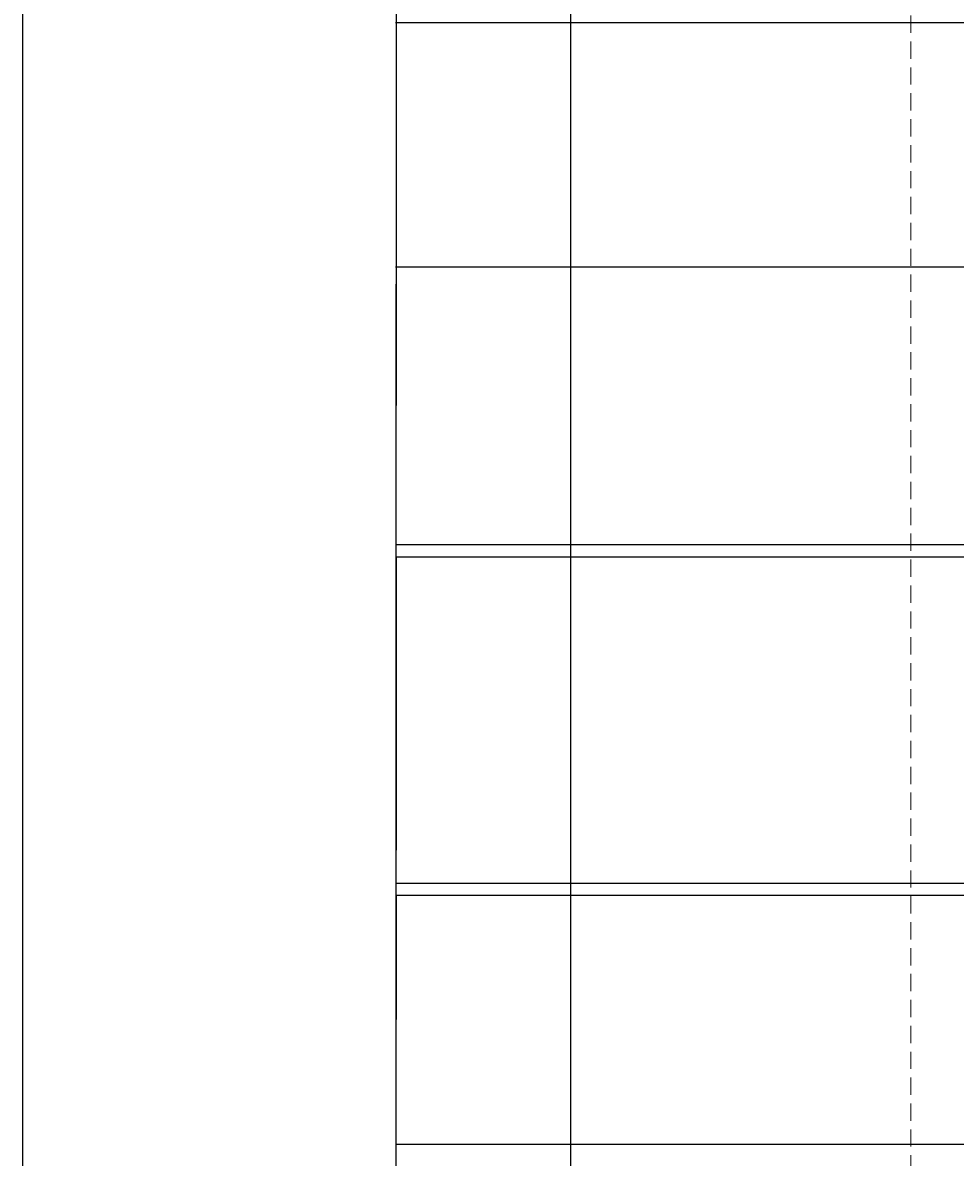
# Model space of a CAD drawing. Units: inches. Extents: x 1770 to 2988, y 1161 to 3221.
# Tile 7 of 44: x 1770 to 2113, y 1614 to 2032. Entities that reach past the tile are written whole.
import ezdxf

# ---------------------------------------------------------------- set-up
doc = ezdxf.new("R2010")
doc.units = ezdxf.units.IN
doc.linetypes.add('DASHED2', pattern=[9.525, 6.35, -3.175])
for name, color, linetype, lineweight in [('A-ANNO-DIMS', 2, 'Continuous', 18), ('A-ANNO-TTLB', 7, 'Continuous', 25), ('A-ROOF-OVHD', 7, 'DASHED2', 18), ('C-PROP', 7, 'Continuous', 25)]:
    doc.layers.add(name, color=color, linetype=linetype, lineweight=lineweight)
doc.styles.get("Standard").update_dxf_attribs({"font": 'arial.ttf'})
doc.dimstyles.get("Standard").update_dxf_attribs({"dimtxt": 0.18, "dimasz": 0.18, "dimexe": 0.18, "dimexo": 0.0625, "dimgap": 0.09, "dimtad": 0, "dimtih": 1, "dimtoh": 1, "dimdec": 4, "dimzin": 0, "dimdsep": 46, "dimtxsty": 'Standard', "dimcen": 0.09, "dimadec": 0, "dimazin": 0, "dimtfac": 1, "dimtdec": 4, "dimtofl": 0, "dimtmove": 0, "dimatfit": 3, "dimfxl": 1, "dimtolj": 1, "dimtzin": 0, "dimarcsym": 0})

# ---------------------------------------------------------------- blocks, each defined once
blk = doc.blocks.new('*D57')
at = {"layer": 'A-ANNO-DIMS', "color": 0, "lineweight": -2, "transparency": 16777216}
for p, q in [((1971.47, 2506.27), (1907.1, 2506.27)), ((1907.28, 2506.09), (1907.28, 1915.08)), ((1907.28, 1323.71), (1907.28, 1914.72)), ((1971.47, 1323.53), (1907.1, 1323.53))]:
    blk.add_line(p, q, dxfattribs=at)
at = {"layer": 'A-ANNO-DIMS', "color": 0, "transparency": 16777216}
for points in [[(1907.25, 2506.09), (1907.31, 2506.09), (1907.28, 2506.27)], [(1907.25, 1323.71), (1907.31, 1323.71), (1907.28, 1323.53)]]:
    blk.add_solid(points, dxfattribs=at)
at = {"layer": 'Defpoints', "color": 0, "transparency": 16777216}
for p in [(1907.28, 2506.27), (1971.53, 2506.27), (1971.53, 1323.53)]:
    blk.add_point(p, dxfattribs=at)
at = {"layer": 'A-ANNO-DIMS', "color": 0, "transparency": 16777216, "insert": (1907.28, 1914.9), "char_height": 0.18, "attachment_point": 5}
blk.add_mtext('\\A1;1182.7', dxfattribs=at)
blk = doc.blocks.new('*D69')
at = {"layer": 'A-ANNO-DIMS', "color": 0, "lineweight": -2, "transparency": 16777216}
for p, q in [((2333.13, 2031.7), (1907.1, 2031.7)), ((1907.28, 2031.52), (1907.28, 1935.88)), ((1907.28, 1839.88), (1907.28, 1935.52)), ((2333.13, 1839.7), (1907.1, 1839.7))]:
    blk.add_line(p, q, dxfattribs=at)
at = {"layer": 'A-ANNO-DIMS', "color": 0, "transparency": 16777216}
for points in [[(1907.25, 2031.52), (1907.31, 2031.52), (1907.28, 2031.7)], [(1907.25, 1839.88), (1907.31, 1839.88), (1907.28, 1839.7)]]:
    blk.add_solid(points, dxfattribs=at)
at = {"layer": 'Defpoints', "color": 0, "transparency": 16777216}
for p in [(1907.28, 2031.7), (2333.2, 2031.7), (2333.2, 1839.7)]:
    blk.add_point(p, dxfattribs=at)
at = {"layer": 'A-ANNO-DIMS', "color": 0, "transparency": 16777216, "insert": (1907.28, 1935.7), "char_height": 0.18, "attachment_point": 5}
blk.add_mtext('\\A1;192', dxfattribs=at)
blk = doc.blocks.new('*D76')
at = {"layer": 'A-ANNO-DIMS', "color": 0, "lineweight": -2, "transparency": 16777216}
for p, q in [((2460.63, 1710.7), (1907.1, 1710.7)), ((1907.28, 1710.52), (1907.28, 1665.13)), ((1907.28, 1619.38), (1907.28, 1664.77)), ((2460.63, 1619.2), (1907.1, 1619.2))]:
    blk.add_line(p, q, dxfattribs=at)
at = {"layer": 'A-ANNO-DIMS', "color": 0, "transparency": 16777216}
for points in [[(1907.25, 1710.52), (1907.31, 1710.52), (1907.28, 1710.7)], [(1907.25, 1619.38), (1907.31, 1619.38), (1907.28, 1619.2)]]:
    blk.add_solid(points, dxfattribs=at)
at = {"layer": 'Defpoints', "color": 0, "transparency": 16777216}
for p in [(1907.28, 1710.7), (2460.7, 1710.7), (2460.7, 1619.2)]:
    blk.add_point(p, dxfattribs=at)
at = {"layer": 'A-ANNO-DIMS', "color": 0, "transparency": 16777216, "insert": (1907.28, 1664.95), "char_height": 0.18, "attachment_point": 5}
blk.add_mtext('\\A1;91.5', dxfattribs=at)
blk = doc.blocks.new('*D78')
at = {"layer": 'A-ANNO-DIMS', "color": 0, "lineweight": -2, "transparency": 16777216}
for p, q in [((2160.63, 1835.2), (1907.1, 1835.2)), ((1907.28, 1835.02), (1907.28, 1727.38)), ((1907.28, 1619.38), (1907.28, 1727.02)), ((2160.63, 1619.2), (1907.1, 1619.2))]:
    blk.add_line(p, q, dxfattribs=at)
at = {"layer": 'A-ANNO-DIMS', "color": 0, "transparency": 16777216}
for points in [[(1907.25, 1835.02), (1907.31, 1835.02), (1907.28, 1835.2)], [(1907.25, 1619.38), (1907.31, 1619.38), (1907.28, 1619.2)]]:
    blk.add_solid(points, dxfattribs=at)
at = {"layer": 'Defpoints', "color": 0, "transparency": 16777216}
for p in [(1907.28, 1835.2), (2160.7, 1835.2), (2160.7, 1619.2)]:
    blk.add_point(p, dxfattribs=at)
at = {"layer": 'A-ANNO-DIMS', "color": 0, "transparency": 16777216, "insert": (1907.28, 1727.2), "char_height": 0.18, "attachment_point": 5}
blk.add_mtext('\\A1;216', dxfattribs=at)
blk = doc.blocks.new('*D83')
at = {"layer": 'A-ANNO-DIMS', "color": 0, "lineweight": -2, "transparency": 16777216}
for p, q in [((2513.13, 1835.2), (1907.1, 1835.2)), ((1907.28, 1835.02), (1907.28, 1775.38)), ((1907.28, 1715.38), (1907.28, 1775.02)), ((2513.13, 1715.2), (1907.1, 1715.2))]:
    blk.add_line(p, q, dxfattribs=at)
at = {"layer": 'A-ANNO-DIMS', "color": 0, "transparency": 16777216}
for points in [[(1907.25, 1835.02), (1907.31, 1835.02), (1907.28, 1835.2)], [(1907.25, 1715.38), (1907.31, 1715.38), (1907.28, 1715.2)]]:
    blk.add_solid(points, dxfattribs=at)
at = {"layer": 'Defpoints', "color": 0, "transparency": 16777216}
for p in [(1907.28, 1835.2), (2513.2, 1835.2), (2513.2, 1715.2)]:
    blk.add_point(p, dxfattribs=at)
at = {"layer": 'A-ANNO-DIMS', "color": 0, "transparency": 16777216, "insert": (1907.28, 1775.2), "char_height": 0.18, "attachment_point": 5}
blk.add_mtext('\\A1;120', dxfattribs=at)
blk = doc.blocks.new('*D90')
at = {"layer": 'A-ANNO-DIMS', "color": 0, "lineweight": -2, "transparency": 16777216}
for p, q in [((2616.63, 1941.8), (1907.1, 1941.8)), ((1907.28, 1941.62), (1907.28, 1890.93)), ((1907.28, 1839.88), (1907.28, 1890.57)), ((2616.63, 1839.7), (1907.1, 1839.7))]:
    blk.add_line(p, q, dxfattribs=at)
at = {"layer": 'A-ANNO-DIMS', "color": 0, "transparency": 16777216}
for points in [[(1907.25, 1941.62), (1907.31, 1941.62), (1907.28, 1941.8)], [(1907.25, 1839.88), (1907.31, 1839.88), (1907.28, 1839.7)]]:
    blk.add_solid(points, dxfattribs=at)
at = {"layer": 'Defpoints', "color": 0, "transparency": 16777216}
for p in [(1907.28, 1941.8), (2616.7, 1941.8), (2616.7, 1839.7)]:
    blk.add_point(p, dxfattribs=at)
at = {"layer": 'A-ANNO-DIMS', "color": 0, "transparency": 16777216, "insert": (1907.28, 1890.75), "char_height": 0.18, "attachment_point": 5}
blk.add_mtext('\\A1;102.1', dxfattribs=at)

msp = doc.modelspace()

# ---------------------------------------------------------------- linework, layer by layer
at = {"layer": 'A-ANNO-TTLB'}
msp.add_lwpolyline([(1769.9155, 3221.2788), (2987.7567, 3221.2788), (2987.7567, 1161.1516), (1769.9155, 1161.1516)], close=True, dxfattribs=at)
at = {"layer": 'A-ROOF-OVHD'}
msp.add_line((2096.7313, 2405.7876), (2096.7313, 1610.2021), dxfattribs=at)
at = {"layer": 'C-PROP'}
msp.add_lwpolyline([(1971.5344, 2506.2747), (2802.4374, 2506.2747), (2802.4374, 1323.5288), (1971.5344, 1323.5288)], close=True, dxfattribs=at)

# ---------------------------------------------------------------- dimensions: what is measured, and where the dimension line sits
at = {"layer": 'A-ANNO-DIMS'}
for base, p1, p2, override, picture, middle in [((1907.2844, 2506.2747), (1971.5344, 1323.5288), (1971.5344, 2506.2747), {"dimdec": 1, "dimlfac": 1, "dimrnd": 0, "dimzin": 0, "dimdsep": 46, "dimlunit": 2}, '*D57', (1907.2844, 1914.9017)), ((1907.2844, 2031.7021), (2333.196, 1839.7021), (2333.196, 2031.7021), {"dimdec": 0, "dimlfac": 1, "dimrnd": 0, "dimzin": 0, "dimdsep": 46, "dimlunit": 2}, '*D69', (1907.2844, 1935.7021)), ((1907.2844, 1941.8004), (2616.696, 1839.7021), (2616.696, 1941.8004), {"dimdec": 1, "dimlfac": 1, "dimrnd": 0, "dimzin": 0, "dimdsep": 46, "dimlunit": 2}, '*D90', (1907.2844, 1890.7512)), ((1907.2844, 1835.2021), (2160.696, 1619.2021), (2160.696, 1835.2021), {"dimdec": 0, "dimlfac": 1, "dimrnd": 0, "dimzin": 0, "dimdsep": 46, "dimlunit": 2}, '*D78', (1907.2844, 1727.2021)), ((1907.2844, 1835.2021), (2513.196, 1715.2021), (2513.196, 1835.2021), {"dimdec": 0, "dimlfac": 1, "dimrnd": 0, "dimzin": 0, "dimdsep": 46, "dimlunit": 2}, '*D83', (1907.2844, 1775.2021)), ((1907.2844, 1710.7021), (2460.696, 1619.2021), (2460.696, 1710.7021), {"dimdec": 1, "dimlfac": 1, "dimrnd": 0, "dimzin": 0, "dimdsep": 46, "dimlunit": 2}, '*D76', (1907.2844, 1664.9521))]:
    dim = msp.add_linear_dim(base=base, p1=p1, p2=p2, angle=90, dimstyle='Standard', override=override, dxfattribs=at)
    dim.commit()
    dim.dimension.update_dxf_attribs({"geometry": picture, "text_midpoint": middle})

doc.saveas('drawing.dxf')
